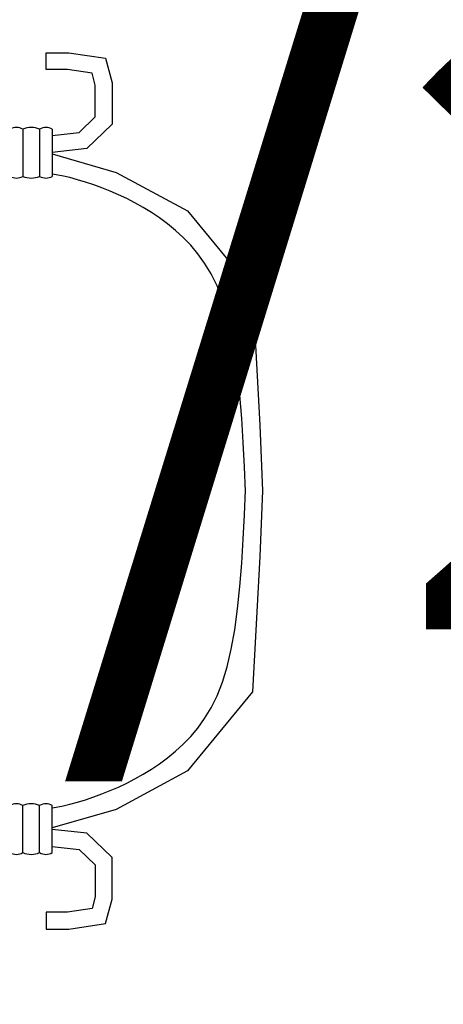
# Model space of a CAD drawing. Units: inches. Extents: x 2278 to 7495, y -71 to 1198.
# Tile 33 of 44: x 5134.27 to 5138.354, y 136.372 to 145.876. Entities that reach past the tile are written whole.
import ezdxf

# ---------------------------------------------------------------- set-up
doc = ezdxf.new("R2010")
doc.units = ezdxf.units.IN
doc.header["$MEASUREMENT"] = 0
doc.layers.add('A-ANNO-DIMS', color=2, linetype='Continuous', lineweight=18)
doc.layers.add('A-ELEV', color=7, linetype='Continuous', lineweight=25)
doc.styles.get("Standard").update_dxf_attribs({"font": 'arial.ttf'})
doc.dimstyles.get("Standard").update_dxf_attribs({"dimtxt": 6, "dimasz": 3, "dimexe": 0.18, "dimexo": 0.0625, "dimgap": 0.09, "dimtad": 0, "dimtih": 1, "dimtoh": 1, "dimdec": 0, "dimzin": 0, "dimdsep": 46, "dimlunit": 3, "dimtxsty": 'Standard', "dimblk": 'ARCHTICK', "dimcen": 0.09, "dimadec": 0, "dimazin": 0, "dimtfac": 1, "dimtdec": 0, "dimtofl": 0, "dimtmove": 0, "dimatfit": 3, "dimfxl": 1, "dimtolj": 1, "dimtzin": 0, "dimarcsym": 0})

# ---------------------------------------------------------------- blocks, each defined once
blk = doc.blocks.new('_ArchTick')
at = {"color": 0, "linetype": 'ByBlock', "const_width": 0.15}
blk.add_lwpolyline([(-0.5, -0.5), (0.5, 0.5)], dxfattribs=at)
blk = doc.blocks.new('*D59')
at = {"layer": 'A-ANNO-DIMS', "color": 0, "lineweight": -2, "transparency": 16777216}
for p, q in [((5096.5894, 159.1826), (5101.5644, 159.1826)), ((5101.3844, 159.1826), (5101.3844, 146.185)), ((5101.3844, 126.7988), (5101.3844, 139.7963)), ((5096.5894, 126.7988), (5101.5644, 126.7988))]:
    blk.add_line(p, q, dxfattribs=at)
at = {"layer": 'Defpoints', "color": 0, "transparency": 16777216}
for p in [(5096.5269, 159.1826), (5101.3844, 159.1826), (5096.5269, 126.7988)]:
    blk.add_point(p, dxfattribs=at)
at = {"layer": 'A-ANNO-DIMS', "color": 0, "lineweight": -2, "transparency": 16777216, "xscale": 3, "yscale": 3, "zscale": 3}
for p, rotation in [((5101.3844, 159.1826), 90), ((5101.3844, 126.7988), 270)]:
    blk.add_blockref('_ArchTick', p, dxfattribs=dict(at, rotation=rotation))
at = {"layer": 'A-ANNO-DIMS', "color": 0, "transparency": 16777216, "insert": (5101.3844, 142.9907), "char_height": 6, "attachment_point": 5}
blk.add_mtext('\\A1;ORNATE BALUSTER 2\'-8 1/2" TYP.', dxfattribs=at)
blk = doc.blocks.new('*D123')
at = {"layer": 'A-ANNO-DIMS', "color": 0, "lineweight": -2, "transparency": 16777216}
for p, q in [((4736.95, 340.1567), (4736.95, -23.4272)), ((5145.6762, -1.8097), (5145.6762, -23.4272)), ((4736.95, -23.2472), (4923.9291, -23.2472)), ((5145.6762, -23.2472), (4958.6971, -23.2472))]:
    blk.add_line(p, q, dxfattribs=at)
at = {"layer": 'Defpoints', "color": 0, "transparency": 16777216}
for p in [(4736.95, 340.2192), (5145.6762, -1.7472), (5145.6762, -23.2472)]:
    blk.add_point(p, dxfattribs=at)
at = {"layer": 'A-ANNO-DIMS', "color": 0, "lineweight": -2, "transparency": 16777216, "xscale": 3, "yscale": 3, "zscale": 3, "rotation": 180}
blk.add_blockref('_ArchTick', (4736.95, -23.2472), dxfattribs=at)
at = {"layer": 'A-ANNO-DIMS', "color": 0, "lineweight": -2, "transparency": 16777216, "xscale": 3, "yscale": 3, "zscale": 3}
blk.add_blockref('_ArchTick', (5145.6762, -23.2472), dxfattribs=at)
at = {"layer": 'A-ANNO-DIMS', "color": 0, "transparency": 16777216, "insert": (4941.3131, -23.2472), "char_height": 6, "attachment_point": 5}
blk.add_mtext('\\A1;34\'-0 1/2"', dxfattribs=at)
blk = doc.blocks.new('*D131')
at = {"layer": 'A-ANNO-DIMS', "color": 0, "lineweight": -2, "transparency": 16777216}
for p, q in [((5096.1762, 99.3153), (5096.1762, 361.8992)), ((5145.6762, 118.3153), (5145.6762, 361.8992)), ((5096.1762, 361.7192), (5105.7503, 361.7192)), ((5145.6762, 361.7192), (5136.1022, 361.7192))]:
    blk.add_line(p, q, dxfattribs=at)
at = {"layer": 'Defpoints', "color": 0, "transparency": 16777216}
for p in [(5145.6762, 361.7192), (5145.6762, 118.2528), (5096.1762, 99.2528)]:
    blk.add_point(p, dxfattribs=at)
at = {"layer": 'A-ANNO-DIMS', "color": 0, "lineweight": -2, "transparency": 16777216, "xscale": 3, "yscale": 3, "zscale": 3, "rotation": 180}
blk.add_blockref('_ArchTick', (5096.1762, 361.7192), dxfattribs=at)
at = {"layer": 'A-ANNO-DIMS', "color": 0, "lineweight": -2, "transparency": 16777216, "xscale": 3, "yscale": 3, "zscale": 3}
blk.add_blockref('_ArchTick', (5145.6762, 361.7192), dxfattribs=at)
at = {"layer": 'A-ANNO-DIMS', "color": 0, "transparency": 16777216, "insert": (5120.9262, 361.7192), "char_height": 6, "attachment_point": 5}
blk.add_mtext('\\A1;4\'-1 1/2"', dxfattribs=at)
blk = doc.blocks.new('*D139')
at = {"layer": 'A-ANNO-DIMS', "color": 0, "lineweight": -2, "transparency": 16777216}
for p, q in [((5092.2387, 160.2528), (5167.7538, 160.2528)), ((5167.5738, 160.2528), (5167.5738, 142.4083)), ((5167.5738, 118.2528), (5167.5738, 136.0973)), ((5145.7387, 118.2528), (5167.7538, 118.2528))]:
    blk.add_line(p, q, dxfattribs=at)
at = {"layer": 'Defpoints', "color": 0, "transparency": 16777216}
for p in [(5092.1762, 160.2528), (5167.5738, 160.2528), (5145.6762, 118.2528)]:
    blk.add_point(p, dxfattribs=at)
at = {"layer": 'A-ANNO-DIMS', "color": 0, "lineweight": -2, "transparency": 16777216, "xscale": 3, "yscale": 3, "zscale": 3}
for p, rotation in [((5167.5738, 160.2528), 90), ((5167.5738, 118.2528), 270)]:
    blk.add_blockref('_ArchTick', p, dxfattribs=dict(at, rotation=rotation))
at = {"layer": 'A-ANNO-DIMS', "color": 0, "transparency": 16777216, "insert": (5167.5738, 139.2528), "char_height": 6, "attachment_point": 5}
blk.add_mtext('\\A1;3\'-6"', dxfattribs=at)

msp = doc.modelspace()

# ---------------------------------------------------------------- linework, layer by layer
at = {"layer": 'A-ELEV'}
for p, q in [((5134.5263, 145.3952), (5134.5263, 145.5581)), ((5134.5263, 145.5581), (5134.7441, 145.5581)), ((5134.7441, 145.5581), (5135.0979, 145.5036)), ((5135.0979, 145.5036), (5135.1614, 145.2675)), ((5134.7316, 145.3952), (5134.5263, 145.3952)), ((5134.9681, 145.3587), (5134.7316, 145.3952)), ((5134.9985, 145.246), (5134.9681, 145.3587)), ((5134.9985, 144.9373), (5134.9985, 145.246)), ((5135.1614, 145.2675), (5135.1614, 144.868)), ((5134.8435, 144.7879), (5134.9985, 144.9373)), ((5135.1614, 144.868), (5134.9164, 144.632)), ((5134.2991, 144.8198), (5134.2991, 144.3639)), ((5134.462, 144.8198), (5134.462, 144.3639)), ((5134.5842, 144.8198), (5134.5842, 144.3639)), ((5134.5842, 144.7597), (5134.8435, 144.7879)), ((5134.9164, 144.632), (5134.5842, 144.5958)), ((5134.5842, 144.581), (5135.1984, 144.402)), ((5134.6032, 144.3836), (5134.5842, 144.3865)), ((5134.6774, 144.3696), (5134.6032, 144.3836)), ((5135.1984, 144.402), (5135.8884, 144.03)), ((5134.7525, 144.3524), (5134.6774, 144.3696)), ((5134.8285, 144.3322), (5134.7525, 144.3524)), ((5134.9054, 144.3089), (5134.8285, 144.3322)), ((5134.9832, 144.2827), (5134.9054, 144.3089)), ((5135.0619, 144.2535), (5134.9832, 144.2827)), ((5135.1415, 144.2214), (5135.0619, 144.2535)), ((5135.2214, 144.1867), (5135.1415, 144.2214)), ((5135.3013, 144.149), (5135.2214, 144.1867)), ((5135.3809, 144.1081), (5135.3013, 144.149)), ((5135.4602, 144.0636), (5135.3809, 144.1081)), ((5135.539, 144.0151), (5135.4602, 144.0636)), ((5135.6172, 143.9622), (5135.539, 144.0151)), ((5135.8884, 144.03), (5136.5149, 143.2679)), ((5135.6947, 143.9045), (5135.6172, 143.9622)), ((5135.7713, 143.8416), (5135.6947, 143.9045)), ((5135.8462, 143.7735), (5135.7713, 143.8416)), ((5135.9185, 143.6994), (5135.8462, 143.7735)), ((5135.9876, 143.6175), (5135.9185, 143.6994)), ((5136.0533, 143.5262), (5135.9876, 143.6175)), ((5136.1151, 143.4234), (5136.0533, 143.5262)), ((5136.1725, 143.3071), (5136.1151, 143.4234)), ((5136.2246, 143.1752), (5136.1725, 143.3071)), ((5136.5149, 143.2679), (5136.5856, 141.9615)), ((5136.2708, 143.0257), (5136.2246, 143.1752)), ((5136.3104, 142.8565), (5136.2708, 143.0257)), ((5136.3437, 142.6689), (5136.3104, 142.8565)), ((5136.3711, 142.466), (5136.3437, 142.6689)), ((5136.3935, 142.2507), (5136.3711, 142.466)), ((5136.4115, 142.0258), (5136.3935, 142.2507)), ((5136.4259, 141.7942), (5136.4115, 142.0258)), ((5136.5856, 141.9615), (5136.6103, 141.3278)), ((5136.4376, 141.5585), (5136.4259, 141.7942)), ((5136.4475, 141.321), (5136.4376, 141.5585)), ((5136.4376, 141.0971), (5136.4475, 141.3345)), ((5136.6103, 141.3278), (5136.5856, 140.694)), ((5136.4259, 140.8614), (5136.4376, 141.0971)), ((5136.4115, 140.6297), (5136.4259, 140.8614)), ((5136.5856, 140.694), (5136.5149, 139.3876)), ((5136.3935, 140.4049), (5136.4115, 140.6297)), ((5136.3711, 140.1895), (5136.3935, 140.4049)), ((5136.3437, 139.9866), (5136.3711, 140.1895)), ((5136.3104, 139.799), (5136.3437, 139.9866)), ((5136.2708, 139.6298), (5136.3104, 139.799)), ((5136.2246, 139.4803), (5136.2708, 139.6298)), ((5136.1725, 139.3484), (5136.2246, 139.4803)), ((5136.5149, 139.3876), (5135.8884, 138.6255)), ((5136.1151, 139.2321), (5136.1725, 139.3484)), ((5136.0533, 139.1293), (5136.1151, 139.2321)), ((5135.9876, 139.038), (5136.0533, 139.1293)), ((5135.9185, 138.9562), (5135.9876, 139.038)), ((5135.7713, 138.8139), (5135.8462, 138.882)), ((5135.8462, 138.882), (5135.9185, 138.9562)), ((5135.6947, 138.751), (5135.7713, 138.8139)), ((5135.539, 138.6404), (5135.6172, 138.6933)), ((5135.6172, 138.6933), (5135.6947, 138.751)), ((5135.8884, 138.6255), (5135.1984, 138.2535)), ((5135.3809, 138.5474), (5135.4602, 138.5919)), ((5135.4602, 138.5919), (5135.539, 138.6404)), ((5135.2214, 138.4689), (5135.3013, 138.5065)), ((5135.3013, 138.5065), (5135.3809, 138.5474)), ((5134.9832, 138.3729), (5135.0619, 138.402)), ((5135.0619, 138.402), (5135.1415, 138.4341)), ((5135.1415, 138.4341), (5135.2214, 138.4689)), ((5134.6774, 138.286), (5134.7525, 138.3031)), ((5134.7525, 138.3031), (5134.8285, 138.3234)), ((5134.8285, 138.3234), (5134.9054, 138.3466)), ((5134.9054, 138.3466), (5134.9832, 138.3729)), ((5134.2991, 137.8357), (5134.2991, 138.2916)), ((5134.462, 137.8357), (5134.462, 138.2916)), ((5134.5842, 137.8357), (5134.5842, 138.2916)), ((5134.5842, 138.2691), (5134.6032, 138.2719)), ((5135.1984, 138.2535), (5134.5842, 138.0746)), ((5134.6032, 138.2719), (5134.6774, 138.286)), ((5134.9164, 138.0235), (5134.5842, 138.0597)), ((5135.1614, 137.7875), (5134.9164, 138.0235)), ((5134.5842, 137.8958), (5134.8435, 137.8676)), ((5134.8435, 137.8676), (5134.9985, 137.7182)), ((5135.1614, 137.388), (5135.1614, 137.7875)), ((5134.9985, 137.7182), (5134.9985, 137.4095)), ((5134.9985, 137.4095), (5134.9681, 137.2968)), ((5135.0979, 137.1519), (5135.1614, 137.388)), ((5134.7316, 137.2604), (5134.5263, 137.2604)), ((5134.5263, 137.2604), (5134.5263, 137.0974)), ((5134.9681, 137.2968), (5134.7316, 137.2604)), ((5134.5263, 137.0974), (5134.7441, 137.0974)), ((5134.7441, 137.0974), (5135.0979, 137.1519))]:
    msp.add_line(p, q, dxfattribs=at)
for centre, radius, start, end in [((5134.238, 144.7149), 0.1214, 59.77678, 120.22322), ((5134.3806, 144.627), 0.2094, 67.10166, 112.89834), ((5134.5231, 144.7149), 0.1214, 59.77678, 120.22322), ((5134.238, 144.4688), 0.1214, 239.77678, 300.22322), ((5134.3806, 144.5568), 0.2094, 247.10166, 292.89834), ((5134.5231, 144.4688), 0.1214, 239.77678, 300.22322), ((5134.238, 138.1867), 0.1214, 59.77678, 120.22322), ((5134.3806, 138.0987), 0.2094, 67.10166, 112.89834), ((5134.5231, 138.1867), 0.1214, 59.77678, 120.22322), ((5134.238, 137.9406), 0.1214, 239.77678, 300.22322), ((5134.3806, 138.0286), 0.2094, 247.10166, 292.89834), ((5134.5231, 137.9406), 0.1214, 239.77678, 300.22322)]:
    msp.add_arc(centre, radius, start, end, dxfattribs=at)

# ---------------------------------------------------------------- dimensions: what is measured, and where the dimension line sits
at = {"layer": 'A-ANNO-DIMS'}
for base, p1, p2, picture, middle in [((5145.6762, 361.7192), (5096.1762, 99.2528), (5145.6762, 118.2528), '*D131', (5120.9262, 361.7192)), ((5145.6762, -23.2472), (4736.95, 340.2192), (5145.6762, -1.7472), '*D123', (4941.3131, -23.2472))]:
    dim = msp.add_linear_dim(base=base, p1=p1, p2=p2, dimstyle='Standard', override={"dimdec": 1, "dimlfac": 1, "dimrnd": 0, "dimzin": 1, "dimdsep": 46, "dimlunit": 4, "dimfrac": 2}, dxfattribs=at)
    dim.commit()
    dim.dimension.update_dxf_attribs({"geometry": picture, "text_midpoint": middle})
dim = msp.add_linear_dim(base=(5101.3844, 159.1826), p1=(5096.5269, 126.7988), p2=(5096.5269, 159.1826), angle=90, text='ORNATE BALUSTER <> TYP.', dimstyle='Standard', override={"dimdec": 1, "dimrnd": 0, "dimzin": 1, "dimlunit": 4, "dimfrac": 2}, dxfattribs=at)
dim.commit()
dim.dimension.update_dxf_attribs({"geometry": '*D59', "text_midpoint": (5101.3844, 142.9907)})
dim = msp.add_linear_dim(base=(5167.5738, 160.2528), p1=(5145.6762, 118.2528), p2=(5092.1762, 160.2528), angle=90, dimstyle='Standard', override={"dimdec": 1, "dimlfac": 1, "dimrnd": 0, "dimzin": 1, "dimdsep": 46, "dimlunit": 4, "dimfrac": 2}, dxfattribs=at)
dim.commit()
dim.dimension.update_dxf_attribs({"geometry": '*D139', "text_midpoint": (5167.5738, 139.2528)})

doc.saveas('drawing.dxf')
